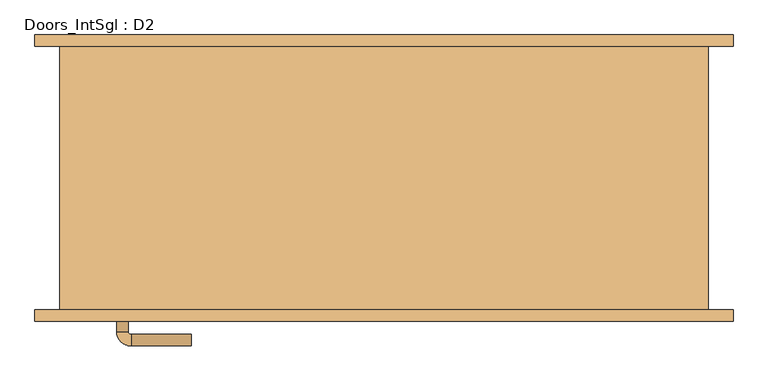
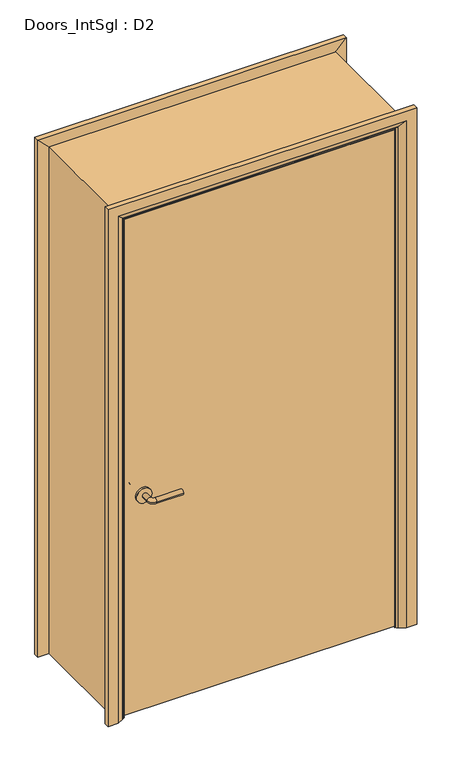
"""IFC4 building model written with IfcOpenShell, lengths in millimetres: door geometry, Doors_IntSgl : D2."""

from ifc_helpers import new_model, si_unit, point, frame, frame_2d, origin, place, context, project, spatial, polyline, circle_curve, ellipse_curve, trimmed, segment, composite_curve, outline, extrude, faceted_brep, source, transform, mapped, element, save
from ifc_brep_helpers import plane_surface, cylinder_surface, revolved_surface, advanced_brep


def doors_intsgl_d2_875133e6(model_context):
    return source(origin(), model_context, "Body", "SolidModel", [
        advanced_brep(
        [(-464.5, -182.6, 900.0), (-444.5, -182.6, 900.0), (-464.5, -152.6, 900.0), (-444.5, -152.6, 900.0), (-439.5, -147.6, 900.0), (-439.5, -127.6, 900.0), (-334.5, -127.6, 900.0), (-334.5, -147.6, 900.0)],
        [
            (0, 1, circle_curve(frame((-454.5, -182.6, 900.0), z_axis=(0.0, -1.0, 0.0), x_axis=(1.0, 0.0, 0.0)), 10.0)),
            (1, 0, circle_curve(frame((-454.5, -182.6, 900.0), z_axis=(0.0, -1.0, 0.0), x_axis=(1.0, 0.0, 0.0)), 10.0)),
            (0, 2),
            (2, 3, circle_curve(frame((-454.5, -152.6, 900.0), z_axis=(0.0, -1.0, 0.0), x_axis=(1.0, 0.0, 0.0)), 10.0)),
            (3, 1),
            (3, 2, circle_curve(frame((-454.5, -152.6, 900.0), z_axis=(0.0, -1.0, 0.0), x_axis=(1.0, 0.0, 0.0)), 10.0)),
            (4, 3, circle_curve(frame((-439.5, -152.6, 900.0), z_axis=(0.0, 0.0, 1.0), x_axis=(-1.0, 0.0, 0.0)), 5.0)),
            (2, 5, circle_curve(frame((-439.5, -152.6, 900.0), z_axis=(0.0, 0.0, -1.0), x_axis=(-1.0, 0.0, 0.0)), 25.0)),
            (5, 4, circle_curve(frame((-439.5, -137.6, 900.0), z_axis=(-1.0, 0.0, 0.0), x_axis=(0.0, -1.0, 0.0)), 10.0)),
            (4, 5, circle_curve(frame((-439.5, -137.6, 900.0), z_axis=(-1.0, 0.0, 0.0), x_axis=(0.0, -1.0, 0.0)), 10.0)),
            (6, 7, circle_curve(frame((-334.5, -137.6, 900.0), z_axis=(1.0, 0.0, 0.0), x_axis=(0.0, -1.0, 0.0)), 10.0)),
            (7, 6, circle_curve(frame((-334.5, -137.6, 900.0), z_axis=(1.0, 0.0, 0.0), x_axis=(0.0, -1.0, 0.0)), 10.0)),
            (5, 6),
            (7, 4),
        ],
        [
            plane_surface(frame((-454.5, -182.6, 900.0), z_axis=(0.0, -1.0, 0.0), x_axis=(0.0, 0.0, 1.0))),
            cylinder_surface(frame((-454.5, -182.6, 900.0), z_axis=(0.0, -1.0, 0.0), x_axis=(1.0, 0.0, 0.0)), 10.0),
            revolved_surface(trimmed(ellipse_curve(frame((-454.5, -152.6, 900.0), z_axis=(0.0, -1.0, 0.0), x_axis=(1.0, 0.0, 0.0)), 10.0, 10.0), [point((-464.5, -152.6, 900.0))], [point((-444.5, -152.6, 900.0))], True, "CARTESIAN"), (-439.5, -152.6, 900.0), (0.0, 0.0, -1.0)),
            revolved_surface(trimmed(ellipse_curve(frame((-454.5, -152.6, 900.0), z_axis=(0.0, -1.0, 0.0), x_axis=(1.0, 0.0, 0.0)), 10.0, 10.0), [point((-444.5, -152.6, 900.0))], [point((-464.5, -152.6, 900.0))], True, "CARTESIAN"), (-439.5, -152.6, 900.0), (0.0, 0.0, -1.0)),
            plane_surface(frame((-334.5, -137.6, 900.0), z_axis=(1.0, 0.0, 0.0), x_axis=(0.0, 0.0, 1.0))),
            cylinder_surface(frame((-439.5, -137.6, 900.0), z_axis=(-1.0, 0.0, 0.0), x_axis=(0.0, -1.0, 0.0)), 10.0),
        ],
        [
            (0, [[1, 2]]),
            (1, [[-1, 3, 4, 5]]),
            (1, [[-2, -5, 6, -3]]),
            (2, [[7, -4, 8, 9]]),
            (3, [[-8, -6, -7, 10]]),
            (4, [[11, 12]]),
            (5, [[-9, 13, -12, 14]]),
            (5, [[-10, -14, -11, -13]]),
        ],
    ),
        extrude(outline(composite_curve([segment(trimmed(circle_curve(frame_2d((900.0, -457.0)), 30.0), [point((900.0, -487.0))], [point((900.0, -427.0))], False, "CARTESIAN"), True, "CONTINUOUS"), segment(trimmed(circle_curve(frame_2d((900.0, -457.0)), 30.0), [point((900.0, -427.0))], [point((900.0, -487.0))], False, "CARTESIAN"), True, "CONTINUOUS")], self_intersect=False)), frame((0.0, -190.6, 0.0), z_axis=(0.0, 1.0, 0.0), x_axis=(0.0, 0.0, 1.0)), (0.0, 0.0, 1.0), 8.0),
        advanced_brep(
        [(-464.5, -236.6, 900.0), (-444.5, -236.6, 900.0), (-444.5, -266.6, 900.0), (-464.5, -266.6, 900.0), (-439.5, -271.6, 900.0), (-439.5, -291.6, 900.0), (-334.5, -291.6, 900.0), (-334.5, -271.6, 900.0)],
        [
            (0, 1, circle_curve(frame((-454.5, -236.6, 900.0), z_axis=(0.0, 1.0, 0.0), x_axis=(1.0, 0.0, 0.0)), 10.0)),
            (1, 0, circle_curve(frame((-454.5, -236.6, 900.0), z_axis=(0.0, 1.0, 0.0), x_axis=(1.0, 0.0, 0.0)), 10.0)),
            (1, 2),
            (2, 3, circle_curve(frame((-454.5, -266.6, 900.0), z_axis=(0.0, 1.0, 0.0), x_axis=(1.0, 0.0, 0.0)), 10.0)),
            (3, 0),
            (3, 2, circle_curve(frame((-454.5, -266.6, 900.0), z_axis=(0.0, 1.0, 0.0), x_axis=(1.0, 0.0, 0.0)), 10.0)),
            (4, 5, circle_curve(frame((-439.5, -281.6, 900.0), z_axis=(-1.0, 0.0, 0.0), x_axis=(0.0, 1.0, 0.0)), 10.0)),
            (5, 3, circle_curve(frame((-439.5, -266.6, 900.0), z_axis=(0.0, 0.0, -1.0), x_axis=(-1.0, 0.0, 0.0)), 25.0)),
            (2, 4, circle_curve(frame((-439.5, -266.6, 900.0), z_axis=(0.0, 0.0, 1.0), x_axis=(-1.0, 0.0, 0.0)), 5.0)),
            (5, 4, circle_curve(frame((-439.5, -281.6, 900.0), z_axis=(-1.0, 0.0, 0.0), x_axis=(0.0, 1.0, 0.0)), 10.0)),
            (6, 7, circle_curve(frame((-334.5, -281.6, 900.0), z_axis=(1.0, 0.0, 0.0), x_axis=(0.0, 1.0, 0.0)), 10.0)),
            (7, 6, circle_curve(frame((-334.5, -281.6, 900.0), z_axis=(1.0, 0.0, 0.0), x_axis=(0.0, 1.0, 0.0)), 10.0)),
            (4, 7),
            (6, 5),
        ],
        [
            plane_surface(frame((-454.5, -236.6, 900.0), z_axis=(0.0, 1.0, 0.0), x_axis=(0.0, 0.0, 1.0))),
            cylinder_surface(frame((-454.5, -236.6, 900.0), z_axis=(0.0, 1.0, 0.0), x_axis=(1.0, 0.0, 0.0)), 10.0),
            revolved_surface(trimmed(ellipse_curve(frame((-454.5, -266.6, 900.0), z_axis=(0.0, -1.0, 0.0), x_axis=(1.0, 0.0, 0.0)), 10.0, 10.0), [point((-464.5, -266.6, 900.0))], [point((-444.5, -266.6, 900.0))], True, "CARTESIAN"), (-439.5, -266.6, 900.0), (0.0, 0.0, -1.0)),
            revolved_surface(trimmed(ellipse_curve(frame((-454.5, -266.6, 900.0), z_axis=(0.0, -1.0, 0.0), x_axis=(1.0, 0.0, 0.0)), 10.0, 10.0), [point((-444.5, -266.6, 900.0))], [point((-464.5, -266.6, 900.0))], True, "CARTESIAN"), (-439.5, -266.6, 900.0), (0.0, 0.0, -1.0)),
            plane_surface(frame((-334.5, -281.6, 900.0), z_axis=(1.0, 0.0, 0.0), x_axis=(0.0, 0.0, 1.0))),
            cylinder_surface(frame((-439.5, -281.6, 900.0), z_axis=(-1.0, 0.0, 0.0), x_axis=(0.0, 1.0, 0.0)), 10.0),
        ],
        [
            (0, [[1, 2]]),
            (1, [[3, 4, 5, -2]]),
            (1, [[-5, 6, -3, -1]]),
            (2, [[7, 8, -4, 9]]),
            (3, [[10, -9, -6, -8]]),
            (4, [[11, 12]]),
            (5, [[13, -11, 14, -7]]),
            (5, [[-14, -12, -13, -10]]),
        ],
    ),
        extrude(outline(composite_curve([segment(trimmed(circle_curve(frame_2d((900.0, -457.0)), 30.0), [point((900.0, -487.0))], [point((900.0, -427.0))], False, "CARTESIAN"), True, "CONTINUOUS"), segment(trimmed(circle_curve(frame_2d((900.0, -457.0)), 30.0), [point((900.0, -427.0))], [point((900.0, -487.0))], False, "CARTESIAN"), True, "CONTINUOUS")], self_intersect=False)), frame((0.0, -236.6, 0.0), z_axis=(0.0, 1.0, 0.0), x_axis=(0.0, 0.0, 1.0)), (0.0, 0.0, 1.0), 8.0),
        extrude(outline(polyline([(529.5, -190.6), (529.5, -228.6), (-529.5, -228.6), (-529.5, -190.6), (529.5, -190.6)])), frame((0.0, 0.0, 8.0), z_axis=(0.0, 0.0, 1.0), x_axis=(1.0, 0.0, 0.0)), (0.0, 0.0, 1.0), 2060.0),
        advanced_brep(
        [(606.5, -248.6, 0.0), (566.5, -248.6, 0.0), (540.5, -234.6, 0.0), (536.5, -228.6, 0.0), (606.5, -228.6, 0.0), (606.5, -228.6, 2145.0), (606.5, -248.6, 2145.0), (536.5, -228.6, 2075.0), (-536.5, -228.6, 2075.0), (-536.5, -228.6, 0.0), (-606.5, -228.6, 0.0), (-606.5, -228.6, 2145.0), (540.5, -234.6, 2079.0), (566.5, -248.6, 2105.0), (-606.5, -248.6, 2145.0), (-606.5, -248.6, 0.0), (-566.5, -248.6, 0.0), (-566.5, -248.6, 2105.0), (-540.5, -234.6, 0.0), (-540.5, -234.6, 2079.0)],
        [
            (0, 1),
            (1, 2),
            (2, 3, circle_curve(frame((544.5, -227.6, 0.0), z_axis=(0.0, 0.0, -1.0), x_axis=(1.0, 0.0, 0.0)), 8.0622577)),
            (3, 4),
            (4, 0),
            (4, 5),
            (5, 6),
            (6, 0),
            (3, 7),
            (7, 8),
            (8, 9),
            (9, 10),
            (10, 11),
            (11, 5),
            (2, 12),
            (12, 7, ellipse_curve(frame((544.5, -227.6, 2083.0), z_axis=(0.7071067811865475, 0.0, -0.7071067811865475), x_axis=(-0.7071067811865474, 0.0, -0.7071067811865476)), 11.4017543, 8.0622577)),
            (1, 13),
            (13, 12),
            (6, 14),
            (14, 15),
            (15, 16),
            (16, 17),
            (17, 13),
            (10, 15),
            (14, 11),
            (9, 18, circle_curve(frame((-544.5, -227.6, 0.0), z_axis=(0.0, 0.0, -1.0), x_axis=(-1.0, 0.0, 0.0)), 8.0622577)),
            (18, 16),
            (19, 18),
            (8, 19, ellipse_curve(frame((-544.5, -227.6, 2083.0), z_axis=(-0.7071067811865475, 0.0, -0.7071067811865475), x_axis=(-0.7071067811865474, 0.0, 0.7071067811865476)), 11.4017543, 8.0622577)),
            (19, 17),
            (12, 19),
        ],
        [
            plane_surface(frame((536.5, -228.6, 0.0), z_axis=(0.0, 0.0, -1.0), x_axis=(0.0, 1.0, 0.0))),
            plane_surface(frame((606.5, -248.6, 0.0), z_axis=(1.0, 0.0, 0.0), x_axis=(0.0, 0.0, 1.0))),
            plane_surface(frame((606.5, -228.6, 0.0), z_axis=(0.0, 1.0, 0.0), x_axis=(0.0, 0.0, 1.0))),
            cylinder_surface(frame((544.5, -227.6, 0.0), z_axis=(0.0, 0.0, -1.0), x_axis=(1.0, 0.0, 0.0)), 8.0622577),
            plane_surface(frame((540.5, -234.6, 0.0), z_axis=(-0.4740998230350126, -0.880471099922178, 0.0), x_axis=(0.0, 0.0, 1.0))),
            plane_surface(frame((566.5, -248.6, 0.0), z_axis=(0.0, -1.0, 0.0), x_axis=(0.0, 0.0, 1.0))),
            plane_surface(frame((-606.5, -248.6, 2145.0), z_axis=(-1.0, 0.0, 0.0), x_axis=(0.0, 0.0, -1.0))),
            plane_surface(frame((-536.5, -228.6, 0.0), z_axis=(0.0, 0.0, -1.0), x_axis=(0.0, 1.0, 0.0))),
            cylinder_surface(frame((-544.5, -227.6, 2075.0), z_axis=(0.0, 0.0, 1.0), x_axis=(-1.0, 0.0, 0.0)), 8.0622577),
            plane_surface(frame((-540.5, -234.6, 2079.0), z_axis=(0.47409982303501824, -0.8804710999221749, 0.0), x_axis=(0.0, 0.0, -1.0))),
            plane_surface(frame((606.5, -248.6, 2145.0), z_axis=(0.0, 0.0, 1.0), x_axis=(-1.0, 0.0, 0.0))),
            cylinder_surface(frame((536.5, -227.6, 2083.0), z_axis=(1.0, 0.0, 0.0), x_axis=(0.0, 0.0, 1.0)), 8.0622577),
            plane_surface(frame((540.5, -234.6, 2079.0), z_axis=(0.0, -0.8804710999221764, -0.4740998230350154), x_axis=(-1.0, 0.0, 0.0))),
        ],
        [
            (0, [[1, 2, 3, 4, 5]]),
            (1, [[6, 7, 8, -5]]),
            (2, [[9, 10, 11, 12, 13, 14, -6, -4]]),
            (3, [[15, 16, -9, -3]]),
            (4, [[17, 18, -15, -2]]),
            (5, [[-8, 19, 20, 21, 22, 23, -17, -1]]),
            (6, [[-13, 24, -20, 25]]),
            (7, [[-24, -12, 26, 27, -21]]),
            (8, [[28, -26, -11, 29]]),
            (9, [[-22, -27, -28, 30]]),
            (10, [[-14, -25, -19, -7]]),
            (11, [[31, -29, -10, -16]]),
            (12, [[-23, -30, -31, -18]]),
        ],
    ),
        extrude(outline(polyline([(0.0, -512.5), (2051.0, -512.5), (2051.0, 512.5), (0.0, 512.5), (0.0, 531.5), (2070.0, 531.5), (2070.0, -531.5), (0.0, -531.5), (0.0, -512.5)])), frame((0.0, -188.6, 0.0), z_axis=(0.0, 1.0, 0.0), x_axis=(0.0, 0.0, 1.0)), (0.0, 0.0, 1.0), 32.0),
        advanced_brep(
        [(-606.5, 248.6, 0.0), (-566.5, 248.6, 0.0), (-540.5, 234.6, 0.0), (-536.5, 228.6, 0.0), (-606.5, 228.6, 0.0), (-606.5, 228.6, 2145.0), (-606.5, 248.6, 2145.0), (-536.5, 228.6, 2075.0), (-540.5, 234.6, 2079.0), (-566.5, 248.6, 2105.0), (606.5, 248.6, 0.0), (606.5, 228.6, 0.0), (536.5, 228.6, 0.0), (540.5, 234.6, 0.0), (566.5, 248.6, 0.0), (606.5, 248.6, 2145.0), (566.5, 248.6, 2105.0), (540.5, 234.6, 2079.0), (536.5, 228.6, 2075.0), (606.5, 228.6, 2145.0)],
        [
            (0, 1),
            (1, 2),
            (2, 3, circle_curve(frame((-544.5, 227.6, 0.0), z_axis=(0.0, 0.0, -1.0), x_axis=(-1.0, 0.0, 0.0)), 8.0622577)),
            (3, 4),
            (4, 0),
            (4, 5),
            (5, 6),
            (6, 0),
            (3, 7),
            (7, 5),
            (2, 8),
            (8, 7, ellipse_curve(frame((-544.5, 227.6, 2083.0), z_axis=(-0.7071067811865475, 0.0, -0.7071067811865475), x_axis=(0.7071067811865474, 0.0, -0.7071067811865476)), 11.4017543, 8.0622577)),
            (1, 9),
            (9, 8),
            (6, 9),
            (10, 11),
            (11, 12),
            (12, 13, circle_curve(frame((544.5, 227.6, 0.0), z_axis=(0.0, 0.0, -1.0), x_axis=(1.0, 0.0, 0.0)), 8.0622577)),
            (13, 14),
            (14, 10),
            (15, 10),
            (14, 16),
            (16, 15),
            (13, 17),
            (17, 16),
            (12, 18),
            (18, 17, ellipse_curve(frame((544.5, 227.6, 2083.0), z_axis=(0.7071067811865475, 0.0, -0.7071067811865475), x_axis=(0.7071067811865474, 0.0, 0.7071067811865476)), 11.4017543, 8.0622577)),
            (11, 19),
            (19, 18),
            (15, 19),
            (5, 19),
            (15, 6),
            (7, 18),
            (8, 17),
            (9, 16),
        ],
        [
            plane_surface(frame((-536.5, 301.4010989, 0.0), z_axis=(0.0, 0.0, -1.0), x_axis=(1.0, 0.0, 0.0))),
            plane_surface(frame((-606.5, 248.6, 0.0), z_axis=(-1.0, 0.0, 0.0), x_axis=(0.0, 0.0, 1.0))),
            plane_surface(frame((-606.5, 228.6, 0.0), z_axis=(0.0, -1.0, 0.0), x_axis=(0.0, 0.0, 1.0))),
            cylinder_surface(frame((-544.5, 227.6, 0.0), z_axis=(0.0, 0.0, -1.0), x_axis=(-1.0, 0.0, 0.0)), 8.0622577),
            plane_surface(frame((-540.5, 234.6, 0.0), z_axis=(0.4740998230350183, 0.8804710999221749, 0.0), x_axis=(0.0, 0.0, 1.0))),
            plane_surface(frame((-566.5, 248.6, 0.0), z_axis=(0.0, 1.0, 0.0), x_axis=(0.0, 0.0, 1.0))),
            plane_surface(frame((536.5, 301.4010989, 0.0), z_axis=(0.0, 0.0, -1.0), x_axis=(-1.0, 0.0, 0.0))),
            plane_surface(frame((566.5, 248.6, 2105.0), z_axis=(0.0, 1.0, 0.0), x_axis=(0.0, 0.0, -1.0))),
            plane_surface(frame((540.5, 234.6, 2079.0), z_axis=(-0.4740998230350183, 0.8804710999221749, 0.0), x_axis=(0.0, 0.0, -1.0))),
            cylinder_surface(frame((544.5, 227.6, 2075.0), z_axis=(0.0, 0.0, 1.0), x_axis=(1.0, 0.0, 0.0)), 8.0622577),
            plane_surface(frame((606.5, 228.6, 2145.0), z_axis=(0.0, -1.0, 0.0), x_axis=(0.0, 0.0, -1.0))),
            plane_surface(frame((606.5, 248.6, 2145.0), z_axis=(1.0, 0.0, 0.0), x_axis=(0.0, 0.0, -1.0))),
            plane_surface(frame((-606.5, 248.6, 2145.0), z_axis=(0.0, 0.0, 1.0), x_axis=(1.0, 0.0, 0.0))),
            plane_surface(frame((-606.5, 228.6, 2145.0), z_axis=(0.0, -1.0, 0.0), x_axis=(1.0, 0.0, 0.0))),
            cylinder_surface(frame((-536.5, 227.6, 2083.0), z_axis=(-1.0, 0.0, 0.0), x_axis=(0.0, 0.0, 1.0)), 8.0622577),
            plane_surface(frame((-540.5, 234.6, 2079.0), z_axis=(0.0, 0.8804710999221749, -0.4740998230350183), x_axis=(1.0, 0.0, 0.0))),
            plane_surface(frame((-566.5, 248.6, 2105.0), z_axis=(0.0, 1.0, 0.0), x_axis=(1.0, 0.0, 0.0))),
        ],
        [
            (0, [[1, 2, 3, 4, 5]]),
            (1, [[6, 7, 8, -5]]),
            (2, [[9, 10, -6, -4]]),
            (3, [[11, 12, -9, -3]]),
            (4, [[13, 14, -11, -2]]),
            (5, [[-8, 15, -13, -1]]),
            (6, [[16, 17, 18, 19, 20]]),
            (7, [[21, -20, 22, 23]]),
            (8, [[-22, -19, 24, 25]]),
            (9, [[-24, -18, 26, 27]]),
            (10, [[-26, -17, 28, 29]]),
            (11, [[-28, -16, -21, 30]]),
            (12, [[31, -30, 32, -7]]),
            (13, [[33, -29, -31, -10]]),
            (14, [[34, -27, -33, -12]]),
            (15, [[35, -25, -34, -14]]),
            (16, [[-32, -23, -35, -15]]),
        ],
    ),
        faceted_brep([(-531.5, -228.6, 0.0), (-563.5, -228.6, 0.0), (-563.5, 228.6, 0.0), (-531.5, 228.6, 0.0), (-531.5, 228.6, 2070.0), (-531.5, -228.6, 2070.0), (-563.5, 228.6, 2102.0), (-563.5, -228.6, 2102.0), (531.5, -228.6, 0.0), (531.5, 228.6, 0.0), (563.5, 228.6, 0.0), (563.5, -228.6, 0.0), (531.5, -228.6, 2070.0), (563.5, -228.6, 2102.0), (563.5, 228.6, 2102.0), (531.5, 228.6, 2070.0)], [[[0, 1, 2, 3]], [[3, 4, 5, 0]], [[2, 6, 4, 3]], [[1, 7, 6, 2]], [[0, 5, 7, 1]], [[8, 9, 10, 11]], [[12, 8, 11, 13]], [[13, 11, 10, 14]], [[14, 10, 9, 15]], [[15, 9, 8, 12]], [[4, 15, 12, 5]], [[6, 14, 15, 4]], [[7, 13, 14, 6]], [[5, 12, 13, 7]]]),
    ])


if __name__ == "__main__":
    model = new_model("IFC4")
    model_context = context("Model", 3, world=origin())
    ifc_project = project(units=[si_unit("LENGTHUNIT", "METRE", prefix="MILLI")], contexts=[model_context])
    site = spatial("IfcSite", under=ifc_project)
    building = spatial("IfcBuilding", under=site)
    placement = place(None, origin())
    doors_intsgl_d2_shape = doors_intsgl_d2_875133e6(model_context)
    element("IfcDoor", 1, ObjectType="Doors_IntSgl : D2", at=placement, inside=building, context=model_context, shape_type="MappedRepresentation", body=[
        mapped(doors_intsgl_d2_shape, transform((0.0, 0.0, 0.0), x_axis=(1.0, 0.0, 0.0), y_axis=(0.0, 1.0, 0.0), z_axis=(0.0, 0.0, 1.0))),
    ])
    save(model, "model.ifc")

# Revit data of these elements
# Type "Doors_IntSgl : D2"
#   Type Mark = "47"
#   Type Comments = "Internal Single"
#   Operation = "SingleSwingRight"
#   Manufacturer = "Revit"
#   Keynote = "L20"
#   Description = "Internal Single Door"
#   Analytic Construction = "Metal"
#   UnderCut = 8 mm
#   Tolerance = 2 mm
#   Thickness = 38 mm
#   Thermal Resistance (R) = 0.270117 (m²·K)/W
#   Structural Tolerance = 8 mm
#   StopDepth = 32 mm
#   Stop Thickness = 19 mm
#   Rough Width = 1143 mm
#   Rough Height = 2110 mm
#   Height to Top Lock Rail = 1000 mm
#   Heat Transfer Coefficient (U) = 3.7021 W/(m²·K)
#   Handle Z Distance = 900 mm
#   Handle X Distance = 75 mm
#   Frame Thickness = 32 mm
#   Door Panel Width = 1059 mm
#   Door Panel Thickness = 38 mm
#   Door Panel Offset = 0 mm
#   Height = 2110 mm
#   Width = 1143 mm
#   Door Panel Height = 2060 mm
#   Architrave Setback = 5 mm
#   Vis - Ironmongery = yes
#   Material Ironmongery = Door - Handle
#   Material Frame = Door - Frame/Mullion (1)
#   Material Door = Door - Panel
#   Material Architrave = Door - Architrave
#   Visual Light Transmittance = 0
#   Solar Heat Gain Coefficient = 0
#   Function = (empty or 0)
#   Wall Closure = (empty or 0)
# Element 1 (IfcDoor, "Doors_IntSgl : D2")
#   Materials on its faces: "Door - Architrave", "Door - Handle", "Door - Frame/Mullion (1)", "Door - Panel"
# Materials
#   "Door - Handle": colour RGB 0 0 0, transparency 0, Keynote = "P21", Cost = 0
#   "Door - Frame/Mullion (1)": class "Wood", colour RGB 212 179 113, transparency 0, Keynote = "L20", Cost = 0
#   "Door - Panel": class "Wood", colour RGB 210 159 95, transparency 0, Keynote = "L20", Cost = 0
#   "Door - Architrave": class "Wood", colour RGB 154 90 5, transparency 0, Keynote = "P20", Cost = 0
